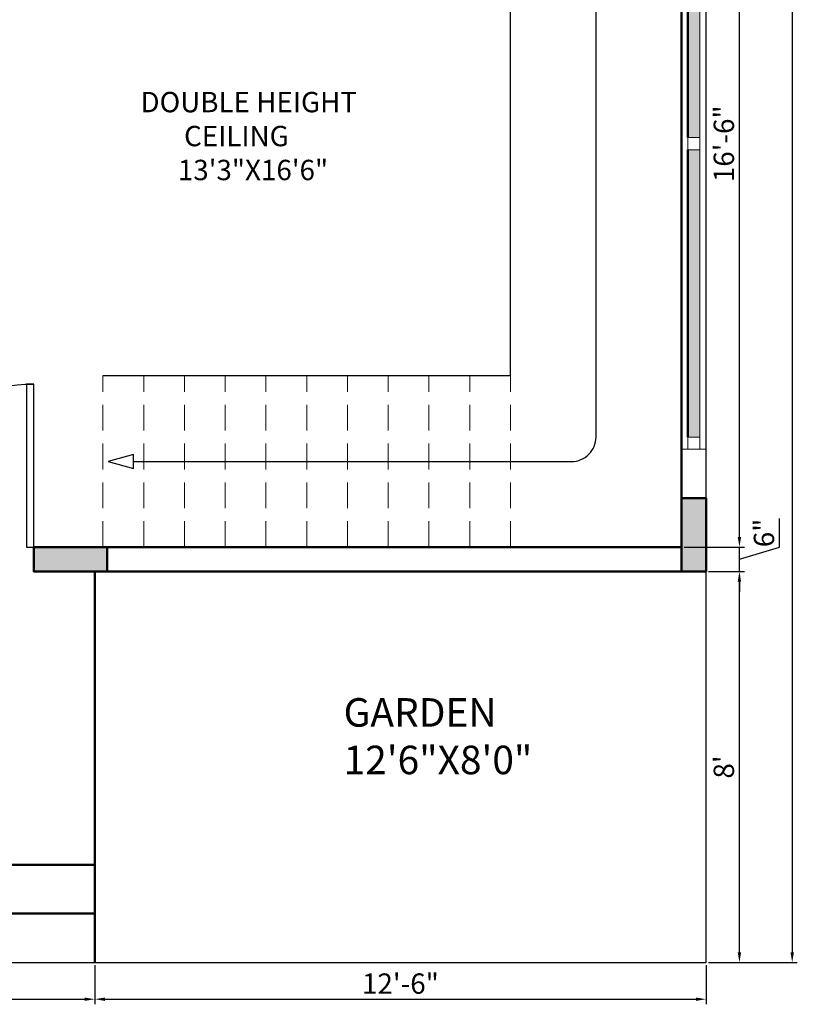
# Model space of a CAD drawing. Units: inches. Extents: x 3064 to 19385, y 846 to 15425.
# Tile 57 of 108: x 6216 to 6407, y 1462 to 1703. Entities that reach past the tile are written whole.
import ezdxf

# ---------------------------------------------------------------- set-up
doc = ezdxf.new("R2010")
doc.units = ezdxf.units.IN
doc.linetypes.add('DASHED', pattern=[19.05, 12.7, -6.35])
for name, color, linetype, lineweight in [('A-ANNO-DIMS', 2, 'Continuous', 18), ('A-AREA-IDEN', 3, 'Continuous', 18), ('A-COLS', 1, 'Continuous', 35), ('A-DOOR', 3, 'Continuous', 25), ('A-FLOR-STRS', 2, 'Continuous', 25), ('A-FLOR-STRS-OVHD', 2, 'DASHED', 18), ('A-GLAZ', 4, 'Continuous', 18), ('A-WALL', 7, 'Continuous', 50), ('C-PROP', 6, 'Continuous', 25)]:
    doc.layers.add(name, color=color, linetype=linetype, lineweight=lineweight)
doc.styles.get("Standard").update_dxf_attribs({"font": 'arial.ttf'})
doc.dimstyles.new('ISO-25', dxfattribs={"dimtxt": 9, "dimasz": 2.5, "dimexe": 1.25, "dimexo": 0.625, "dimtad": 1, "dimdec": 1, "dimlunit": 3, "dimtxsty": 'Standard', "dimcen": 2.5, "dimadec": 0, "dimazin": 0, "dimtfac": 1, "dimtdec": 1, "dimtmove": 0, "dimatfit": 3, "dimfxl": 1, "dimarcsym": 0})

# ---------------------------------------------------------------- blocks, each defined once
blk = doc.blocks.new('*U2')
for p, q in [((0, 0), (0, -6)), ((40, 0), (40, -6))]:
    blk.add_line(p, q)
blk.add_lwpolyline([(0, 0), (0, 40), (1.75, 40), (1.75, 0)], close=True)
blk.add_arc((0, 0), 40, 0, 90)
blk = doc.blocks.new('*D355')
at = {"layer": 'A-ANNO-DIMS', "color": 0, "lineweight": -2, "transparency": 16777216}
for p, q in [((6042.49, 1471.36), (6042.49, 1461.73)), ((6234.49, 1471.36), (6234.49, 1461.73)), ((6044.99, 1462.98), (6231.99, 1462.98))]:
    blk.add_line(p, q, dxfattribs=at)
at = {"layer": 'A-ANNO-DIMS', "color": 0, "transparency": 16777216}
for points in [[(6044.99, 1463.39), (6044.99, 1462.56), (6042.49, 1462.98)], [(6231.99, 1463.39), (6231.99, 1462.56), (6234.49, 1462.98)]]:
    blk.add_solid(points, dxfattribs=at)
at = {"layer": 'Defpoints', "color": 0, "transparency": 16777216}
for p in [(6042.49, 1471.99), (6234.49, 1471.99), (6234.49, 1462.98)]:
    blk.add_point(p, dxfattribs=at)
at = {"layer": 'A-ANNO-DIMS', "color": 0, "transparency": 16777216, "insert": (6138.49, 1466.16), "char_height": 5, "attachment_point": 5}
blk.add_mtext("16'", dxfattribs=at)
blk = doc.blocks.new('*D356')
at = {"layer": 'A-ANNO-DIMS', "color": 0, "lineweight": -2, "transparency": 16777216}
for p, q in [((6234.49, 1471.36), (6234.49, 1461.73)), ((6384.49, 1471.36), (6384.49, 1461.73)), ((6236.99, 1462.98), (6381.99, 1462.98))]:
    blk.add_line(p, q, dxfattribs=at)
at = {"layer": 'A-ANNO-DIMS', "color": 0, "transparency": 16777216}
for points in [[(6236.99, 1463.39), (6236.99, 1462.56), (6234.49, 1462.98)], [(6381.99, 1463.39), (6381.99, 1462.56), (6384.49, 1462.98)]]:
    blk.add_solid(points, dxfattribs=at)
at = {"layer": 'Defpoints', "color": 0, "transparency": 16777216}
for p in [(6234.49, 1471.99), (6384.49, 1471.99), (6384.49, 1462.98)]:
    blk.add_point(p, dxfattribs=at)
at = {"layer": 'A-ANNO-DIMS', "color": 0, "transparency": 16777216, "insert": (6309.49, 1466.16), "char_height": 5, "attachment_point": 5}
blk.add_mtext('12\'-6"', dxfattribs=at)
blk = doc.blocks.new('*D357')
at = {"layer": 'A-ANNO-DIMS', "color": 0, "lineweight": -2, "transparency": 16777216}
for p, q in [((6385.12, 1567.99), (6393.94, 1567.99)), ((6392.69, 1474.49), (6392.69, 1565.49)), ((6385.12, 1471.99), (6393.94, 1471.99))]:
    blk.add_line(p, q, dxfattribs=at)
at = {"layer": 'A-ANNO-DIMS', "color": 0, "transparency": 16777216}
for points in [[(6392.27, 1565.49), (6393.1, 1565.49), (6392.69, 1567.99)], [(6392.27, 1474.49), (6393.1, 1474.49), (6392.69, 1471.99)]]:
    blk.add_solid(points, dxfattribs=at)
at = {"layer": 'Defpoints', "color": 0, "transparency": 16777216}
for p in [(6384.49, 1567.99), (6392.69, 1567.99), (6384.49, 1471.99)]:
    blk.add_point(p, dxfattribs=at)
at = {"layer": 'A-ANNO-DIMS', "color": 0, "transparency": 16777216, "insert": (6389.51, 1519.99), "char_height": 5, "attachment_point": 5, "rotation": 90}
blk.add_mtext("8'", dxfattribs=at)
blk = doc.blocks.new('*D358')
at = {"layer": 'A-ANNO-DIMS', "color": 0, "lineweight": -2, "transparency": 16777216}
for p, q in [((6402.53, 1573.94), (6402.53, 1580.97)), ((6392.69, 1576.49), (6392.69, 1578.99)), ((6379.12, 1573.99), (6393.94, 1573.99)), ((6392.69, 1567.99), (6392.69, 1573.99)), ((6392.69, 1567.99), (6392.69, 1573.99)), ((6392.69, 1570.99), (6402.53, 1573.94)), ((6385.12, 1567.99), (6393.94, 1567.99)), ((6392.69, 1565.49), (6392.69, 1562.99))]:
    blk.add_line(p, q, dxfattribs=at)
at = {"layer": 'A-ANNO-DIMS', "color": 0, "transparency": 16777216}
for points in [[(6392.27, 1576.49), (6393.1, 1576.49), (6392.69, 1573.99)], [(6392.27, 1565.49), (6393.1, 1565.49), (6392.69, 1567.99)]]:
    blk.add_solid(points, dxfattribs=at)
at = {"layer": 'Defpoints', "color": 0, "transparency": 16777216}
for p in [(6378.49, 1573.99), (6392.69, 1573.99), (6384.49, 1567.99)]:
    blk.add_point(p, dxfattribs=at)
at = {"layer": 'A-ANNO-DIMS', "color": 0, "transparency": 16777216, "insert": (6399.35, 1577.45), "char_height": 5, "attachment_point": 5, "rotation": 90}
blk.add_mtext('6"', dxfattribs=at)
blk = doc.blocks.new('*D350')
at = {"layer": 'A-ANNO-DIMS', "color": 0, "lineweight": -2, "transparency": 16777216}
for p, q in [((6379.12, 1771.99), (6393.94, 1771.99)), ((6392.69, 1576.49), (6392.69, 1769.49)), ((6379.12, 1573.99), (6393.94, 1573.99))]:
    blk.add_line(p, q, dxfattribs=at)
at = {"layer": 'A-ANNO-DIMS', "color": 0, "transparency": 16777216}
for points in [[(6392.27, 1769.49), (6393.1, 1769.49), (6392.69, 1771.99)], [(6392.27, 1576.49), (6393.1, 1576.49), (6392.69, 1573.99)]]:
    blk.add_solid(points, dxfattribs=at)
at = {"layer": 'Defpoints', "color": 0, "transparency": 16777216}
for p in [(6378.49, 1771.99), (6392.69, 1771.99), (6378.49, 1573.99)]:
    blk.add_point(p, dxfattribs=at)
at = {"layer": 'A-ANNO-DIMS', "color": 0, "transparency": 16777216, "insert": (6389.51, 1672.99), "char_height": 5, "attachment_point": 5, "rotation": 90}
blk.add_mtext('16\'-6"', dxfattribs=at)
blk = doc.blocks.new('*D377')
at = {"layer": 'A-ANNO-DIMS', "color": 0, "lineweight": -2, "transparency": 16777216}
for p, q in [((6385.12, 1987.99), (6406.89, 1987.99)), ((6405.64, 1985.49), (6405.64, 1474.49)), ((6385.12, 1471.99), (6406.89, 1471.99))]:
    blk.add_line(p, q, dxfattribs=at)
at = {"layer": 'A-ANNO-DIMS', "color": 0, "transparency": 16777216}
for points in [[(6405.22, 1985.49), (6406.05, 1985.49), (6405.64, 1987.99)], [(6405.22, 1474.49), (6406.05, 1474.49), (6405.64, 1471.99)]]:
    blk.add_solid(points, dxfattribs=at)
at = {"layer": 'Defpoints', "color": 0, "transparency": 16777216}
for p in [(6384.49, 1987.99), (6384.49, 1471.99), (6405.64, 1471.99)]:
    blk.add_point(p, dxfattribs=at)
at = {"layer": 'A-ANNO-DIMS', "color": 0, "transparency": 16777216, "insert": (6402.46, 1729.99), "char_height": 5, "attachment_point": 5, "rotation": 90}
blk.add_mtext("43'", dxfattribs=at)
blk = doc.blocks.new('WIN-1800-PAIR')
h = blk.add_hatch(color=256)
h.dxf.hatch_style = 1
h.paths.add_polyline_path([(0, 0), (3, 0), (3, 70.5), (0, 70.5)])
h.paths.add_polyline_path([(3, 144), (0, 144), (0, 73.5), (3, 73.5)])
blk.add_line((3, 144), (3, 73.5))
blk.add_lwpolyline([(3, 144), (0, 144), (0, 147), (3, 147)], close=True)
blk = doc.blocks.new('WIN-2000')
blk.add_line((3, 0), (3, 70.5))
blk.add_lwpolyline([(3, 70.5), (0, 70.5), (0, 73.5), (3, 73.5)], close=True)

msp = doc.modelspace()

# ---------------------------------------------------------------- hatches: boundary and pattern name
at = {"layer": 'A-COLS'}
h = msp.add_hatch(color=256, dxfattribs=at)
h.dxf.hatch_style = 1
h.paths.add_polyline_path([(6378.49, 1567.99), (6384.49, 1567.99), (6384.49, 1585.99), (6378.49, 1585.99)])
h = msp.add_hatch(color=256, dxfattribs=at)
h.dxf.hatch_style = 1
h.paths.add_polyline_path([(6237.49, 1567.99), (6237.49, 1573.99), (6219.49, 1573.99), (6219.49, 1567.99)])

# ---------------------------------------------------------------- linework, layer by layer
at = {"layer": 'A-FLOR-STRS'}
for q in [(6336.49, 1771.99), (6236.49, 1615.99)]:
    msp.add_line((6336.49, 1615.99), q, dxfattribs=at)
msp.add_lwpolyline([(6243.98, 1594.99), (6351.49, 1594.99, 0.414214), (6357.49, 1600.99), (6357.49, 1744.99, 0.414214), (6351.49, 1750.99), (6224.49, 1750.99)], format="xyb", dxfattribs=at)
msp.add_lwpolyline([(6237.79, 1594.99), (6243.98, 1593.26), (6243.98, 1596.72)], close=True, dxfattribs=at)
at = {"layer": 'A-FLOR-STRS-OVHD', "ltscale": 0.5}
for p, q in [((6236.49, 1573.99), (6236.49, 1615.99)), ((6246.49, 1573.99), (6246.49, 1615.99)), ((6256.49, 1573.99), (6256.49, 1615.99)), ((6266.49, 1573.99), (6266.49, 1615.99)), ((6276.49, 1573.99), (6276.49, 1615.99)), ((6286.49, 1573.99), (6286.49, 1615.99)), ((6296.49, 1573.99), (6296.49, 1615.99)), ((6306.49, 1573.99), (6306.49, 1615.99)), ((6316.49, 1573.99), (6316.49, 1615.99)), ((6326.49, 1573.99), (6326.49, 1615.99)), ((6336.49, 1573.99), (6336.49, 1615.99))]:
    msp.add_line(p, q, dxfattribs=at)
at = {"layer": 'A-GLAZ'}
msp.add_line((6384.49, 1597.99), (6378.49, 1597.99), dxfattribs=at)
msp.add_line((6384.49, 1597.99), (6378.49, 1597.99), dxfattribs=at)
msp.add_lwpolyline([(6382.99, 1597.99), (6379.99, 1597.99), (6379.99, 1600.99), (6382.99, 1600.99)], close=True, dxfattribs=at)
at = {"layer": 'A-WALL'}
for p, q in [((6378.49, 1573.99), (6378.49, 1771.99)), ((6379.99, 1744.99), (6379.99, 1674.49)), ((6379.99, 1600.99), (6379.99, 1671.49)), ((6378.49, 1573.99), (6219.49, 1573.99)), ((6219.49, 1567.99), (6219.49, 1573.99)), ((6384.49, 1567.99), (6219.49, 1567.99)), ((6234.49, 1567.99), (6234.49, 1471.99)), ((6042.49, 1495.99), (6234.49, 1495.99)), ((6042.49, 1483.99), (6234.49, 1483.99))]:
    msp.add_line(p, q, dxfattribs=at)
for points in [[(6384.49, 1567.99), (6384.49, 1585.99), (6378.49, 1585.99), (6378.49, 1567.99)], [(6237.49, 1573.99), (6219.49, 1573.99), (6219.49, 1567.99), (6237.49, 1567.99)]]:
    msp.add_lwpolyline(points, close=True, dxfattribs=at)
at = {"layer": 'C-PROP'}
for p, q in [((6384.49, 1471.99), (6384.49, 1987.99)), ((6042.49, 1471.99), (6384.49, 1471.99))]:
    msp.add_line(p, q, dxfattribs=at)

# ---------------------------------------------------------------- block references
at = {"layer": 'A-DOOR', "xscale": -1}
msp.add_blockref('*U2', (6219.49, 1573.99), dxfattribs=at)
at = {"layer": 'A-GLAZ'}
for name in ['WIN-1800-PAIR', 'WIN-2000']:
    msp.add_blockref(name, (6379.99, 1600.99), dxfattribs=at)

# ---------------------------------------------------------------- texts
at = {"layer": 'A-AREA-IDEN', "attachment_point": 1}
for s, width, insert, char_height in [('DOUBLE HEIGHT \\P       CEILING            \\P      13\'3"X16\'6"', 57.0817, (6245.7, 1685.72), 5), ('GARDEN\\P12\'6"X8\'0"', 67.5924, (6295.54, 1536.89), 7)]:
    msp.add_mtext_dynamic_manual_height_columns(s, width=width, gutter_width=12.5, heights=[0], dxfattribs=dict(at, insert=insert, char_height=char_height))

# ---------------------------------------------------------------- dimensions: what is measured, and where the dimension line sits
at = {"layer": 'A-ANNO-DIMS'}
for base, p1, p2, override, picture, middle in [((6405.64, 1471.99), (6384.49, 1987.99), (6384.49, 1471.99), {"dimtxt": 5, "dimclrd": 0, "dimclre": 0, "dimclrt": 0}, '*D377', (6402.46, 1729.99)), ((6392.69, 1771.99), (6378.49, 1573.99), (6378.49, 1771.99), {"dimtxt": 5, "dimclrd": 0, "dimclre": 0, "dimclrt": 0, "dimtmove": 1}, '*D350', (6389.51, 1672.99)), ((6392.69, 1573.99), (6384.49, 1567.99), (6378.49, 1573.99), {"dimtxt": 5, "dimclrd": 0, "dimclre": 0, "dimclrt": 0, "dimtmove": 1}, '*D358', (6399.35, 1574.57)), ((6392.69, 1567.99), (6384.49, 1471.99), (6384.49, 1567.99), {"dimtxt": 5, "dimclrd": 0, "dimclre": 0, "dimclrt": 0}, '*D357', (6389.51, 1519.99))]:
    dim = msp.add_linear_dim(base=base, p1=p1, p2=p2, angle=90, dimstyle='ISO-25', override=override, dxfattribs=at)
    dim.commit()
    dim.dimension.update_dxf_attribs({"geometry": picture, "text_midpoint": middle})
for base, p1, p2, override, picture, middle in [((6234.49, 1462.98), (6042.49, 1471.99), (6234.49, 1471.99), {"dimtxt": 5, "dimclrd": 0, "dimclre": 0, "dimclrt": 0}, '*D355', (6138.49, 1466.16)), ((6384.49, 1462.98), (6234.49, 1471.99), (6384.49, 1471.99), {"dimtxt": 5, "dimclrd": 0, "dimclre": 0, "dimclrt": 0, "dimtmove": 1}, '*D356', (6309.49, 1466.16))]:
    dim = msp.add_linear_dim(base=base, p1=p1, p2=p2, dimstyle='ISO-25', override=override, dxfattribs=at)
    dim.commit()
    dim.dimension.update_dxf_attribs({"geometry": picture, "text_midpoint": middle})

doc.saveas('drawing.dxf')
